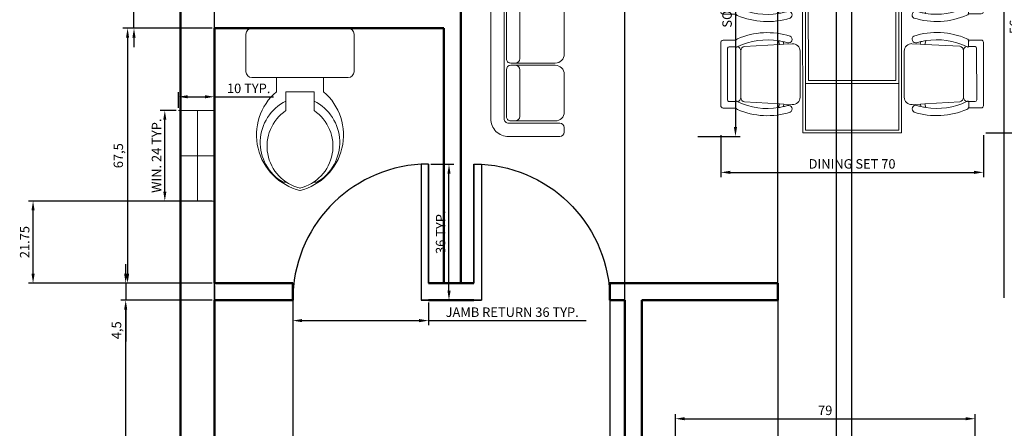
# Model space of a CAD drawing. Units: inches. Extents: x 907 to 2409, y 377 to 1163.
# Tile 2 of 9: x 936 to 1197, y 579 to 687. Entities that reach past the tile are written whole.
import ezdxf

# ---------------------------------------------------------------- set-up
doc = ezdxf.new("R2010")
doc.units = ezdxf.units.IN
for name, color, linetype, lineweight in [('A-ANNO-DIMS', 2, 'Continuous', 18), ('A-DOOR', 3, 'Continuous', 25), ('A-FLOR-FIXT', 9, 'Continuous', 18), ('A-FURN', 8, 'Continuous', 18), ('A-GLAZ', 4, 'Continuous', 18), ('A-WALL', 7, 'Continuous', 50)]:
    doc.layers.add(name, color=color, linetype=linetype, lineweight=lineweight)
doc.styles.get("Standard").update_dxf_attribs({"font": 'arial.ttf'})
doc.dimstyles.new('ISO-25', dxfattribs={"dimtxt": 2.5, "dimasz": 2.5, "dimexe": 1.25, "dimexo": 0.625, "dimtad": 1, "dimtxsty": 'Standard', "dimcen": 2.5, "dimadec": 0, "dimazin": 0, "dimtfac": 1, "dimtmove": 0, "dimatfit": 3, "dimfxl": 1, "dimarcsym": 0})

# ---------------------------------------------------------------- blocks, each defined once
blk = doc.blocks.new('A$C02F3725D')
for p, q in [((0.025, 0.69), (0.435, 0.69)), ((0, 0.505), (0, 0.665)), ((0.46, 0.665), (0.46, 0.505)), ((0.435, 0.48), (0.025, 0.48)), ((0.13, 0.48), (0.13, 0.42)), ((0.33, 0.42), (0.33, 0.48)), ((0.17, 0.34), (0.17, 0.42)), ((0.17, 0.42), (0.29, 0.42)), ((0.29, 0.34), (0.29, 0.42)), ((0.1578, 0.035), (0.1724, 0.035)), ((0.2876, 0.035), (0.3022, 0.035))]:
    blk.add_line(p, q)
for centre, radius, start, end in [((0.025, 0.665), 0.025, 90, 180), ((0.435, 0.665), 0.025, 0, 90), ((0.025, 0.505), 0.025, 180, 270), ((0.435, 0.505), 0.025, 270, 0), ((0.2874, 0.2356), 0.2425, 130.4885, 256.2965), ((0.1726, 0.2356), 0.2425, 283.7035, 49.5115), ((0.2568, 0.2042), 0.196, 116.2742, 239.6668), ((0.2032, 0.2042), 0.196, 300.3332, 63.7258), ((0.2732, 0.1883), 0.1834, 124.2157, 256.394), ((0.1868, 0.1883), 0.1834, 283.606, 55.7843)]:
    blk.add_arc(centre, radius, start, end)
blk = doc.blocks.new('A$C2AFA021D')
for p, q in [((0.8, 2.3), (0.2, 2.3)), ((0.85, 2.2), (0.85, 2.25)), ((0.2, 2.15), (0.8, 2.15)), ((0.225, 2.125), (0.275, 2.125)), ((0.75, 2.125), (0.275, 2.125)), ((0, 2.1), (0, 0.2)), ((0.15, 0.2), (0.15, 2.1)), ((0.175, 1.55), (0.175, 2.075)), ((0.325, 2.075), (0.325, 1.55)), ((0.85, 1.6), (0.85, 2.025)), ((0.275, 1.5), (0.225, 1.5)), ((0.225, 1.475), (0.275, 1.475)), ((0.275, 1.5), (0.75, 1.5)), ((0.75, 1.475), (0.275, 1.475)), ((0.175, 0.875), (0.175, 1.425)), ((0.325, 1.425), (0.325, 0.875)), ((0.85, 0.925), (0.85, 1.375)), ((0.275, 0.825), (0.225, 0.825)), ((0.225, 0.8), (0.275, 0.8)), ((0.275, 0.825), (0.75, 0.825)), ((0.75, 0.8), (0.275, 0.8)), ((0.975, 0.825), (1.4, 0.825)), ((1.625, 0.825), (2.075, 0.825)), ((2.3, 0.825), (2.725, 0.825)), ((2.85, 0.2), (2.85, 0.775)), ((2.9, 0.825), (2.95, 0.825)), ((3, 0.775), (3, 0.2)), ((0.175, 0.225), (0.175, 0.75)), ((0.325, 0.75), (0.325, 0.225)), ((0.85, 0.275), (0.85, 0.7)), ((0.875, 0.275), (0.875, 0.725)), ((1.5, 0.725), (1.5, 0.275)), ((1.525, 0.275), (1.525, 0.725)), ((2.175, 0.725), (2.175, 0.275)), ((2.2, 0.275), (2.2, 0.725)), ((2.825, 0.725), (2.825, 0.275)), ((0.875, 0.275), (0.875, 0.225)), ((1.45, 0.325), (0.925, 0.325)), ((1.5, 0.225), (1.5, 0.275)), ((1.525, 0.275), (1.525, 0.225)), ((2.125, 0.325), (1.575, 0.325)), ((2.175, 0.225), (2.175, 0.275)), ((2.2, 0.275), (2.2, 0.225)), ((2.775, 0.325), (2.25, 0.325)), ((2.825, 0.225), (2.825, 0.275)), ((0.8, 0.15), (0.2, 0.15)), ((0.275, 0.175), (0.225, 0.175)), ((0.275, 0.175), (0.75, 0.175)), ((0.925, 0.175), (1.45, 0.175)), ((0.925, 0.15), (2.8, 0.15)), ((1.575, 0.175), (2.125, 0.175)), ((2.25, 0.175), (2.775, 0.175)), ((0.85, 0), (0.85, 0.1)), ((0.875, 0.1), (0.875, 0)), ((0.2, 0), (0.85, 0)), ((2.8, 0), (0.875, 0))]:
    blk.add_line(p, q)
for centre, radius, start, end in [((0.2, 2.1), 0.2, 90, 180), ((0.8, 2.25), 0.05, 0, 90), ((0.2, 2.1), 0.05, 90, 180), ((0.225, 2.075), 0.05, 90, 180), ((0.275, 2.075), 0.05, 0, 90), ((0.75, 2.025), 0.1, 0, 90), ((0.8, 2.2), 0.05, 270, 0), ((0.225, 1.55), 0.05, 180, 270), ((0.275, 1.55), 0.05, 270, 0), ((0.75, 1.6), 0.1, 270, 0), ((0.225, 1.425), 0.05, 90, 180), ((0.275, 1.425), 0.05, 0, 90), ((0.75, 1.375), 0.1, 360, 90), ((0.75, 0.925), 0.1, 270, 0), ((0.225, 0.875), 0.05, 180, 270), ((0.225, 0.75), 0.05, 90, 180), ((0.275, 0.875), 0.05, 270, 0), ((0.275, 0.75), 0.05, 0, 90), ((0.75, 0.7), 0.1, 0, 90), ((0.975, 0.725), 0.1, 90, 180), ((1.4, 0.725), 0.1, 0, 90), ((1.625, 0.725), 0.1, 90, 180), ((2.075, 0.725), 0.1, 0, 90), ((2.3, 0.725), 0.1, 90, 180), ((2.725, 0.725), 0.1, 0, 90), ((2.9, 0.775), 0.05, 90, 180), ((2.95, 0.775), 0.05, 0, 90), ((0.225, 0.225), 0.05, 180, 270), ((0.275, 0.225), 0.05, 270, 0), ((0.75, 0.275), 0.1, 270, 0), ((0.925, 0.275), 0.05, 90, 180), ((0.925, 0.225), 0.05, 180, 270), ((1.45, 0.275), 0.05, 360, 90), ((1.45, 0.225), 0.05, 270, 0), ((1.575, 0.275), 0.05, 90, 180), ((1.575, 0.225), 0.05, 180, 270), ((2.125, 0.275), 0.05, 360, 90), ((2.125, 0.225), 0.05, 270, 0), ((2.25, 0.275), 0.05, 90, 180), ((2.25, 0.225), 0.05, 180, 270), ((2.775, 0.275), 0.05, 360, 90), ((2.775, 0.225), 0.05, 270, 0), ((0.2, 0.2), 0.2, 180, 270), ((0.2, 0.2), 0.05, 180, 270), ((0.8, 0.1), 0.05, 0, 90), ((0.925, 0.1), 0.05, 90, 180), ((2.8, 0.2), 0.2, 270, 0), ((2.8, 0.2), 0.05, 270, 0)]:
    blk.add_arc(centre, radius, start, end)
blk = doc.blocks.new('A$C7D96336B')
for p, q in [((280, 0.2), (-280, -0.2)), ((280.8, -1199.8), (280, 0.2)), ((-280, -0.2), (-279.2, -1200.2)), ((264, -15.8), (-264, -16.2)), ((-264, -16.2), (-263.2, -1184.2)), ((264.8, -1183.8), (264, -15.8)), ((-742.8, -515.1), (-743.2, -156.2)), ((-658.1, -143.4), (-730.7, -143.6)), ((-659.8, -143.4), (-659.7, -178.7)), ((-416.5, -146.3), (-411.5, -167.3)), ((-386.1, -165.8), (-411.5, -167.3)), ((-389.5, -151.7), (-386.1, -165.8)), ((-338.9, -163.1), (-386.1, -165.8)), ((339.1, -162.6), (386.3, -165.3)), ((389.7, -151.1), (386.3, -165.3)), ((386.3, -165.3), (411.7, -166.7)), ((416.7, -145.7), (411.7, -166.7)), ((411.7, -166.7), (609.3, -177.8)), ((658.3, -142.5), (730.9, -142.6)), ((659.9, -142.6), (659.9, -177.8)), ((743.5, -514.1), (743.4, -155.2)), ((-704.9, -188.8), (-704.6, -482.3)), ((-659.3, -180.3), (-696.6, -180.5)), ((-629.9, -467.6), (-630.2, -203.4)), ((-411.5, -167.3), (-609.1, -178.7)), ((-294.5, -465.7), (-294.4, -204.7)), ((295.2, -465.3), (294.7, -204.3)), ((630.5, -466.8), (630.5, -202.5)), ((659.5, -179.5), (696.9, -179.5)), ((705.2, -187.9), (705.3, -481.4)), ((-263.8, -280.2), (264.2, -279.8)), ((-263.8, -280.2), (264.2, -279.8)), ((-263.4, -920.2), (-263.8, -280.2)), ((-247.8, -296.2), (248.2, -295.8)), ((-247.4, -904.2), (-247.8, -296.2)), ((248.2, -295.8), (248.6, -903.8)), ((264.2, -279.8), (264.6, -919.8)), ((-659, -490.7), (-696.3, -490.7)), ((-659.4, -522.3), (-659.3, -492.4)), ((-411.1, -503.3), (-608.7, -492.3)), ((411.8, -502.7), (609.4, -491.4)), ((659.6, -489.8), (697, -489.7)), ((660.1, -521.4), (660, -491.5)), ((-657.7, -527.6), (-730.3, -527.6)), ((-416.1, -524.3), (-411.1, -503.3)), ((-385.8, -504.7), (-411.1, -503.3)), ((-389.1, -518.8), (-385.8, -504.7)), ((-338.5, -507.3), (-385.8, -504.7)), ((339.2, -506.9), (386.5, -504.2)), ((386.5, -504.2), (411.8, -502.7)), ((389.8, -518.3), (386.5, -504.2)), ((416.8, -523.7), (411.8, -502.7)), ((658.4, -526.7), (731, -526.6)), ((-742.7, -688.4), (-742.6, -1047.3)), ((-657.6, -675.8), (-730.2, -675.9)), ((-704.4, -1014.6), (-704.5, -721.1)), ((-658.8, -712.7), (-696.2, -712.8)), ((-659.3, -681), (-659.2, -711)), ((-411, -699.8), (-608.6, -711)), ((-416, -678.8), (-411, -699.8)), ((-385.6, -698.3), (-411, -699.8)), ((-389, -684.2), (-385.6, -698.3)), ((-338.4, -695.6), (-385.6, -698.3)), ((339.3, -695.2), (386.6, -697.8)), ((389.9, -683.7), (386.6, -697.8)), ((386.6, -697.8), (411.9, -699.2)), ((416.9, -678.2), (411.9, -699.2)), ((411.9, -699.2), (609.5, -710.2)), ((658.5, -674.9), (731.1, -674.9)), ((659.8, -711.8), (697.1, -711.8)), ((660.2, -680.2), (660.2, -710.1)), ((705.8, -1013.7), (705.5, -720.2)), ((743.6, -687.4), (744, -1046.3)), ((-629.7, -735.7), (-629.6, -1000)), ((-294.4, -737.1), (-293.9, -998.2)), ((295.3, -736.7), (295.2, -997.8)), ((630.7, -734.9), (631, -999.1)), ((264.6, -919.8), (-263.4, -920.2)), ((248.6, -903.8), (-247.4, -904.2)), ((-658.7, -1023), (-696.1, -1023)), ((-659.1, -1059.9), (-659.1, -1024.7)), ((-410.9, -1035.8), (-608.5, -1024.6)), ((-415.9, -1056.8), (-410.9, -1035.8)), ((-385.5, -1037.2), (-410.9, -1035.8)), ((-388.9, -1051.4), (-385.5, -1037.2)), ((-338.3, -1039.9), (-385.5, -1037.2)), ((339.7, -1039.4), (386.9, -1036.7)), ((386.9, -1036.7), (412.3, -1035.2)), ((390.3, -1050.8), (386.9, -1036.7)), ((412.3, -1035.2), (609.9, -1023.8)), ((417.3, -1056.2), (412.3, -1035.2)), ((658.9, -1059), (731.5, -1058.9)), ((660.1, -1022.1), (697.4, -1022)), ((660.6, -1059), (660.5, -1023.8)), ((-657.5, -1059.9), (-730.1, -1059.9)), ((-279.2, -1200.2), (280.8, -1199.8)), ((-263.2, -1184.2), (264.8, -1183.8))]:
    blk.add_line(p, q)
for centre, radius, start, end in [((-478.6, -532.7), 432.3, 72.7119, 113.3258), ((479.4, -532), 432.3, 66.7517, 107.3656), ((-730.7, -156.1), 12.5, 141.7605, 180.1459), ((-730.7, -156.1), 12.5, 90.1463, 141.7605), ((-643.2, -151), 16.7, 153.004, 184.8567), ((-643.2, -151), 16.7, 113.3258, 153.004), ((-479.1, -531.9), 390.7, 80.7703, 115.5809), ((-479.1, -531.9), 390.7, 76.7336, 80.7703), ((-479.1, -531.9), 390.7, 73.1676, 76.7336), ((-360.6, -137.9), 20.8, 254.7795, 60.0186), ((-336.5, -204.7), 41.7, 0.1463, 93.3068), ((336.7, -204.2), 41.7, 86.7707, 179.9312), ((360.7, -137.4), 20.8, 120.0589, 285.298), ((479.9, -531.2), 390.7, 103.3439, 106.9099), ((479.9, -531.2), 390.7, 99.3072, 103.3439), ((479.9, -531.2), 390.7, 64.4966, 99.3072), ((643.4, -150.1), 16.7, 27.0735, 66.7517), ((643.4, -150.1), 16.7, 355.2209, 27.0735), ((730.9, -155.1), 12.5, 38.317, 89.9312), ((730.9, -155.1), 12.5, 359.9316, 38.317), ((-696.6, -188.8), 8.33, 90.1463, 180.1463), ((-655.5, -178.6), 4.17, 180.1463, 296.5296), ((-479.1, -531.9), 390.7, 115.5809, 116.5296), ((-655.2, -203.4), 25, 0.1463, 72.8968), ((-605.2, -203.4), 25, 98.9209, 179.9714), ((605.5, -202.6), 25, 0.1061, 81.1566), ((655.5, -202.5), 25, 107.1807, 179.9312), ((479.9, -531.2), 390.7, 63.5479, 64.4966), ((655.7, -177.8), 4.17, 243.5479, 359.9312), ((696.9, -187.8), 8.33, 359.9312, 89.9312), ((-696.3, -482.3), 8.33, 179.9714, 269.9714), ((-655.2, -492.4), 4.17, 63.5881, 179.9714), ((-479.5, -138.8), 390.7, 243.5881, 244.5368), ((-654.9, -467.6), 25, 287.2209, 359.9714), ((-479.5, -138.8), 390.7, 244.5368, 279.3474), ((-604.9, -467.6), 25, 180.1463, 261.1967), ((-336.2, -465.7), 41.7, 266.8108, 359.9714), ((336.8, -465.3), 41.7, 180.1061, 273.2667), ((479.7, -138.1), 390.7, 260.7301, 295.5407), ((605.5, -466.7), 25, 278.8808, 359.9312), ((655.5, -466.7), 25, 180.1061, 252.8566), ((479.7, -138.1), 390.7, 295.5407, 296.4894), ((655.8, -491.5), 4.17, 0.1061, 116.4894), ((697, -481.4), 8.33, 270.1061, 0.1061), ((-730.3, -515.1), 12.5, 179.9717, 218.3572), ((-730.3, -515.1), 12.5, 218.3572, 269.9714), ((-642.9, -520), 16.7, 175.261, 207.1136), ((-642.9, -520), 16.7, 207.1136, 246.7919), ((-479.1, -138), 432.3, 246.7919, 287.4058), ((-479.5, -138.8), 390.7, 279.3474, 283.3841), ((-479.5, -138.8), 390.7, 283.3841, 286.9501), ((-360.2, -532.5), 20.8, 300.0991, 105.3382), ((360.9, -532), 20.8, 74.7393, 239.9785), ((479.2, -137.3), 432.3, 252.6717, 293.2857), ((479.7, -138.1), 390.7, 253.1274, 256.6934), ((479.7, -138.1), 390.7, 256.6934, 260.7301), ((643.6, -519.1), 16.7, 293.2857, 332.9639), ((643.6, -519.1), 16.7, 332.9639, 4.8165), ((731, -514.1), 12.5, 270.1061, 321.7203), ((731, -514.1), 12.5, 321.7203, 0.1058), ((-642.7, -683.3), 16.7, 113.2857, 152.9639), ((-478.4, -1065.1), 432.3, 72.6717, 113.2857), ((-360.1, -670.4), 20.8, 254.7393, 59.9785), ((361, -670), 20.8, 120.0991, 285.3382), ((479.9, -1064.5), 432.3, 66.7919, 107.4058), ((643.7, -682.5), 16.7, 27.1136, 66.7919), ((-730.2, -688.4), 12.5, 141.7203, 180.1058), ((-730.2, -688.4), 12.5, 90.1061, 141.7203), ((-696.1, -721.1), 8.33, 90.1061, 180.1061), ((-642.7, -683.3), 16.7, 152.9639, 184.8165), ((-655, -711), 4.17, 180.1061, 296.4894), ((-478.9, -1064.3), 390.7, 115.5407, 116.4894), ((-478.9, -1064.3), 390.7, 80.7301, 115.5407), ((-654.7, -735.8), 25, 0.1061, 72.8566), ((-604.7, -735.7), 25, 98.8808, 179.9312), ((-478.9, -1064.3), 390.7, 76.6934, 80.7301), ((-478.9, -1064.3), 390.7, 73.1274, 76.6934), ((-336, -737.2), 41.7, 0.1061, 93.2667), ((337, -736.8), 41.7, 86.8108, 179.9714), ((480.4, -1063.7), 390.7, 103.3841, 106.9501), ((480.4, -1063.7), 390.7, 99.3474, 103.3841), ((480.4, -1063.7), 390.7, 64.5368, 99.3474), ((605.7, -734.9), 25, 0.1463, 81.1967), ((655.7, -734.9), 25, 107.2209, 179.9714), ((480.4, -1063.7), 390.7, 63.5881, 64.5368), ((656, -710.1), 4.17, 243.5881, 359.9714), ((643.7, -682.5), 16.7, 355.261, 27.1136), ((697.1, -720.1), 8.33, 359.9714, 89.9714), ((731.1, -687.4), 12.5, 38.3572, 89.9714), ((731.1, -687.4), 12.5, 359.9717, 38.3572), ((-654.6, -1000), 25, 287.1807, 359.9312), ((-604.6, -999.9), 25, 180.1061, 261.1566), ((-335.9, -998.3), 41.7, 266.7707, 359.9312), ((337.3, -997.8), 41.7, 180.1463, 273.3068), ((606, -999.1), 25, 278.9209, 359.9714), ((656, -999.1), 25, 180.1463, 252.8968), ((-730.1, -1047.4), 12.5, 179.9316, 218.317), ((-730.1, -1047.4), 12.5, 218.317, 269.9312), ((-696.1, -1014.6), 8.33, 179.9312, 269.9312), ((-642.6, -1052.4), 16.7, 175.2209, 207.0735), ((-654.9, -1024.7), 4.17, 63.5479, 179.9312), ((-479.1, -671.2), 390.7, 243.5479, 244.4966), ((-479.1, -671.2), 390.7, 244.4966, 279.3072), ((-479.1, -671.2), 390.7, 279.3072, 283.3439), ((-479.1, -671.2), 390.7, 283.3439, 286.9099), ((-359.9, -1065.1), 20.8, 300.0589, 105.298), ((361.4, -1064.6), 20.8, 74.7795, 240.0186), ((480, -670.6), 390.7, 253.1676, 256.7336), ((480, -670.6), 390.7, 256.7336, 260.7703), ((480, -670.6), 390.7, 260.7703, 295.5809), ((480, -670.6), 390.7, 295.5809, 296.5296), ((644, -1051.5), 16.7, 293.3258, 333.004), ((656.3, -1023.8), 4.17, 0.1463, 116.5296), ((644, -1051.5), 16.7, 333.004, 4.8567), ((697.4, -1013.7), 8.33, 270.1463, 0.1463), ((731.5, -1046.4), 12.5, 270.1463, 321.7605), ((731.5, -1046.4), 12.5, 321.7605, 0.1459), ((-642.6, -1052.4), 16.7, 207.0735, 246.7517), ((-478.6, -670.4), 432.3, 246.7517, 287.3656), ((479.5, -669.8), 432.3, 252.7119, 293.3258)]:
    blk.add_arc(centre, radius, start, end)
blk = doc.blocks.new('*D34')
at = {"layer": 'A-ANNO-DIMS', "color": 0, "lineweight": -2, "transparency": 16777216}
for p, q in [((966.32, 691.62), (966.32, 700.04)), ((986.99, 689.12), (965.07, 689.12)), ((966.32, 684.62), (966.32, 689.12)), ((986.99, 684.62), (965.07, 684.62)), ((966.32, 682.12), (966.32, 679.62))]:
    blk.add_line(p, q, dxfattribs=at)
at = {"layer": 'A-ANNO-DIMS', "color": 0, "transparency": 16777216}
for points in [[(965.9, 691.62), (966.74, 691.62), (966.32, 689.12)], [(965.9, 682.12), (966.74, 682.12), (966.32, 684.62)]]:
    blk.add_solid(points, dxfattribs=at)
at = {"layer": 'Defpoints', "color": 0, "transparency": 16777216}
for p in [(966.32, 689.12), (987.61, 689.12), (987.61, 684.62)]:
    blk.add_point(p, dxfattribs=at)
at = {"layer": 'A-ANNO-DIMS', "color": 0, "transparency": 16777216, "insert": (964.2, 697.08), "char_height": 2.5, "attachment_point": 5, "rotation": 90}
blk.add_mtext('4,5', dxfattribs=at)
blk = doc.blocks.new('*D35')
at = {"layer": 'A-ANNO-DIMS', "color": 0, "lineweight": -2, "transparency": 16777216}
for p, q in [((986.99, 684.62), (963.37, 684.62)), ((964.62, 682.12), (964.62, 619.62)), ((986.99, 617.12), (963.37, 617.12))]:
    blk.add_line(p, q, dxfattribs=at)
at = {"layer": 'A-ANNO-DIMS', "color": 0, "transparency": 16777216}
for points in [[(964.2, 682.12), (965.03, 682.12), (964.62, 684.62)], [(964.2, 619.62), (965.03, 619.62), (964.62, 617.12)]]:
    blk.add_solid(points, dxfattribs=at)
at = {"layer": 'Defpoints', "color": 0, "transparency": 16777216}
for p in [(987.61, 684.62), (964.62, 617.12), (987.61, 617.12)]:
    blk.add_point(p, dxfattribs=at)
at = {"layer": 'A-ANNO-DIMS', "color": 0, "transparency": 16777216, "insert": (962.49, 650.87), "char_height": 2.5, "attachment_point": 5, "rotation": 90}
blk.add_mtext('67,5', dxfattribs=at)
blk = doc.blocks.new('*D36')
at = {"layer": 'A-ANNO-DIMS', "color": 0, "lineweight": -2, "transparency": 16777216}
for p, q in [((964.12, 619.62), (964.12, 622.12)), ((986.99, 617.12), (962.87, 617.12)), ((964.12, 617.12), (964.12, 612.62)), ((986.99, 612.62), (962.87, 612.62)), ((964.12, 610.12), (964.12, 601.7))]:
    blk.add_line(p, q, dxfattribs=at)
at = {"layer": 'A-ANNO-DIMS', "color": 0, "transparency": 16777216}
for points in [[(963.7, 619.62), (964.53, 619.62), (964.12, 617.12)], [(963.7, 610.12), (964.53, 610.12), (964.12, 612.62)]]:
    blk.add_solid(points, dxfattribs=at)
at = {"layer": 'Defpoints', "color": 0, "transparency": 16777216}
for p in [(987.61, 617.12), (964.12, 612.62), (987.61, 612.62)]:
    blk.add_point(p, dxfattribs=at)
at = {"layer": 'A-ANNO-DIMS', "color": 0, "transparency": 16777216, "insert": (962, 604.66), "char_height": 2.5, "attachment_point": 5, "rotation": 90}
blk.add_mtext('4,5', dxfattribs=at)
blk = doc.blocks.new('*D37')
at = {"layer": 'A-ANNO-DIMS', "color": 0, "lineweight": -2, "transparency": 16777216}
for p, q in [((986.99, 612.62), (962.87, 612.62)), ((964.12, 428.37), (964.12, 610.12)), ((986.99, 425.87), (962.87, 425.87))]:
    blk.add_line(p, q, dxfattribs=at)
at = {"layer": 'A-ANNO-DIMS', "color": 0, "transparency": 16777216}
for points in [[(963.7, 610.12), (964.53, 610.12), (964.12, 612.62)], [(963.7, 428.37), (964.53, 428.37), (964.12, 425.87)]]:
    blk.add_solid(points, dxfattribs=at)
at = {"layer": 'Defpoints', "color": 0, "transparency": 16777216}
for p in [(964.12, 612.62), (987.61, 612.62), (987.61, 425.87)]:
    blk.add_point(p, dxfattribs=at)
at = {"layer": 'A-ANNO-DIMS', "color": 0, "transparency": 16777216, "insert": (961.99, 519.25), "char_height": 2.5, "attachment_point": 5, "rotation": 90}
blk.add_mtext('186,75', dxfattribs=at)
blk = doc.blocks.new('WIN-24IN')
for p, q in [((0.53, 23.99), (0, 23.99)), ((9.53, 24), (0.53, 24)), ((5.03, 0), (5.03, 24)), ((9.53, 12), (0.53, 12)), ((9.53, 0), (0.53, 0))]:
    blk.add_line(p, q)
blk = doc.blocks.new('DOOR-36IN-JAMB-RETURN')
for p, q in [((36, 36), (36, 4.5)), ((36, 0), (34, 0)), ((36, 0), (34, 0))]:
    blk.add_line(p, q)
blk.add_lwpolyline([(36, 4.5), (36, 36), (34, 36), (34, 0), (36, 0)])
blk.add_arc((36.06, 0), 36.06, 93.2732, 180)
blk = doc.blocks.new('*D45')
at = {"layer": 'A-ANNO-DIMS', "color": 0, "lineweight": -2, "transparency": 16777216}
for p, q in [((1008.36, 612), (1008.36, 605.97)), ((1044.36, 612), (1044.36, 605.97)), ((1010.86, 607.22), (1041.86, 607.22)), ((1044.36, 607.22), (1086.14, 607.22))]:
    blk.add_line(p, q, dxfattribs=at)
at = {"layer": 'A-ANNO-DIMS', "color": 0, "transparency": 16777216}
for points in [[(1010.86, 607.64), (1010.86, 606.8), (1008.36, 607.22)], [(1041.86, 607.64), (1041.86, 606.8), (1044.36, 607.22)]]:
    blk.add_solid(points, dxfattribs=at)
at = {"layer": 'Defpoints', "color": 0, "transparency": 16777216}
for p in [(1008.36, 612.62), (1044.36, 612.62), (1044.36, 607.22)]:
    blk.add_point(p, dxfattribs=at)
at = {"layer": 'A-ANNO-DIMS', "color": 0, "transparency": 16777216, "insert": (1066.5, 609.12), "char_height": 2.5, "attachment_point": 5}
blk.add_mtext('JAMB RETURN 36 TYP.', dxfattribs=at)
blk = doc.blocks.new('*D46')
at = {"layer": 'A-ANNO-DIMS', "color": 0, "lineweight": -2, "transparency": 16777216}
for p, q in [((1044.99, 648.62), (1051.01, 648.62)), ((1049.76, 615.12), (1049.76, 646.12)), ((1044.99, 612.62), (1051.01, 612.62))]:
    blk.add_line(p, q, dxfattribs=at)
at = {"layer": 'A-ANNO-DIMS', "color": 0, "transparency": 16777216}
for points in [[(1049.35, 646.12), (1050.18, 646.12), (1049.76, 648.62)], [(1049.35, 615.12), (1050.18, 615.12), (1049.76, 612.62)]]:
    blk.add_solid(points, dxfattribs=at)
at = {"layer": 'Defpoints', "color": 0, "transparency": 16777216}
for p in [(1044.36, 648.62), (1049.76, 648.62), (1044.36, 612.62)]:
    blk.add_point(p, dxfattribs=at)
at = {"layer": 'A-ANNO-DIMS', "color": 0, "transparency": 16777216, "insert": (1047.86, 630.62), "char_height": 2.5, "attachment_point": 5, "rotation": 90}
blk.add_mtext('36 TYP.', dxfattribs=at)
blk = doc.blocks.new('*D47')
at = {"layer": 'A-ANNO-DIMS', "color": 0, "lineweight": -2, "transparency": 16777216}
for p, q in [((977.46, 662.87), (973.23, 662.87)), ((974.48, 641.37), (974.48, 660.37)), ((977.46, 638.87), (973.23, 638.87))]:
    blk.add_line(p, q, dxfattribs=at)
at = {"layer": 'A-ANNO-DIMS', "color": 0, "transparency": 16777216}
for points in [[(974.07, 660.37), (974.9, 660.37), (974.48, 662.87)], [(974.07, 641.37), (974.9, 641.37), (974.48, 638.87)]]:
    blk.add_solid(points, dxfattribs=at)
at = {"layer": 'Defpoints', "color": 0, "transparency": 16777216}
for p in [(974.48, 662.87), (978.08, 662.87), (978.08, 638.87)]:
    blk.add_point(p, dxfattribs=at)
at = {"layer": 'A-ANNO-DIMS', "color": 0, "transparency": 16777216, "insert": (972.6, 650.87), "char_height": 2.5, "attachment_point": 5, "rotation": 90}
blk.add_mtext('WIN. 24 TYP.', dxfattribs=at)
blk = doc.blocks.new('*D48')
at = {"layer": 'A-ANNO-DIMS', "color": 0, "lineweight": -2, "transparency": 16777216}
for p, q in [((978.08, 663.5), (978.08, 667.72)), ((987.61, 663.5), (987.61, 667.72)), ((980.58, 666.47), (985.11, 666.47)), ((987.61, 666.47), (1003.3, 666.47))]:
    blk.add_line(p, q, dxfattribs=at)
at = {"layer": 'A-ANNO-DIMS', "color": 0, "transparency": 16777216}
for points in [[(980.58, 666.89), (980.58, 666.05), (978.08, 666.47)], [(985.11, 666.89), (985.11, 666.05), (987.61, 666.47)]]:
    blk.add_solid(points, dxfattribs=at)
at = {"layer": 'Defpoints', "color": 0, "transparency": 16777216}
for p in [(987.61, 666.47), (978.08, 662.87), (987.61, 662.87)]:
    blk.add_point(p, dxfattribs=at)
at = {"layer": 'A-ANNO-DIMS', "color": 0, "transparency": 16777216, "insert": (996.7, 668.37), "char_height": 2.5, "attachment_point": 5}
blk.add_mtext('10 TYP.', dxfattribs=at)
blk = doc.blocks.new('*D53')
at = {"layer": 'A-ANNO-DIMS', "color": 0, "lineweight": -2, "transparency": 16777216}
for p, q in [((1115.67, 726.66), (1126.9, 726.66)), ((1125.65, 724.16), (1125.65, 658.44)), ((1115.67, 655.94), (1126.9, 655.94))]:
    blk.add_line(p, q, dxfattribs=at)
at = {"layer": 'A-ANNO-DIMS', "color": 0, "transparency": 16777216}
for points in [[(1125.24, 724.16), (1126.07, 724.16), (1125.65, 726.66)], [(1125.24, 658.44), (1126.07, 658.44), (1125.65, 655.94)]]:
    blk.add_solid(points, dxfattribs=at)
at = {"layer": 'Defpoints', "color": 0, "transparency": 16777216}
for p in [(1115.05, 726.66), (1115.05, 655.94), (1125.65, 655.94)]:
    blk.add_point(p, dxfattribs=at)
at = {"layer": 'A-ANNO-DIMS', "color": 0, "transparency": 16777216, "insert": (1123.74, 691.3), "char_height": 2.5, "attachment_point": 5, "rotation": 90}
blk.add_mtext('SOFA 71', dxfattribs=at)
blk = doc.blocks.new('*D56')
at = {"layer": 'A-ANNO-DIMS', "color": 0, "lineweight": -2, "transparency": 16777216}
for p, q in [((1109.72, 566.33), (1109.72, 582.49)), ((1189.13, 566.33), (1189.13, 582.49)), ((1112.22, 581.24), (1186.63, 581.24))]:
    blk.add_line(p, q, dxfattribs=at)
at = {"layer": 'A-ANNO-DIMS', "color": 0, "transparency": 16777216}
for points in [[(1112.22, 581.66), (1112.22, 580.83), (1109.72, 581.24)], [(1186.63, 581.66), (1186.63, 580.83), (1189.13, 581.24)]]:
    blk.add_solid(points, dxfattribs=at)
at = {"layer": 'Defpoints', "color": 0, "transparency": 16777216}
for p in [(1189.13, 581.24), (1109.72, 565.7), (1189.13, 565.7)]:
    blk.add_point(p, dxfattribs=at)
at = {"layer": 'A-ANNO-DIMS', "color": 0, "transparency": 16777216, "insert": (1149.42, 583.14), "char_height": 2.5, "attachment_point": 5}
blk.add_mtext('79', dxfattribs=at)
blk = doc.blocks.new('*D57')
at = {"layer": 'A-ANNO-DIMS', "color": 0, "lineweight": -2, "transparency": 16777216}
for p, q in [((1121.75, 656.27), (1121.75, 645.21)), ((1191.34, 656.27), (1191.34, 645.21)), ((1124.25, 646.46), (1188.84, 646.46))]:
    blk.add_line(p, q, dxfattribs=at)
at = {"layer": 'A-ANNO-DIMS', "color": 0, "transparency": 16777216}
for points in [[(1124.25, 646.88), (1124.25, 646.04), (1121.75, 646.46)], [(1188.84, 646.88), (1188.84, 646.04), (1191.34, 646.46)]]:
    blk.add_solid(points, dxfattribs=at)
at = {"layer": 'Defpoints', "color": 0, "transparency": 16777216}
for p in [(1121.75, 656.9), (1191.34, 656.9), (1191.34, 646.46)]:
    blk.add_point(p, dxfattribs=at)
at = {"layer": 'A-ANNO-DIMS', "color": 0, "transparency": 16777216, "insert": (1156.54, 648.38), "char_height": 2.5, "attachment_point": 5}
blk.add_mtext('DINING SET 70', dxfattribs=at)
blk = doc.blocks.new('*D58')
at = {"layer": 'A-ANNO-DIMS', "color": 0, "lineweight": -2, "transparency": 16777216}
for p, q in [((1191.96, 713.06), (1203.02, 713.06)), ((1201.77, 659.4), (1201.77, 710.56)), ((1191.96, 656.9), (1203.02, 656.9))]:
    blk.add_line(p, q, dxfattribs=at)
at = {"layer": 'A-ANNO-DIMS', "color": 0, "transparency": 16777216}
for points in [[(1201.36, 710.56), (1202.19, 710.56), (1201.77, 713.06)], [(1201.36, 659.4), (1202.19, 659.4), (1201.77, 656.9)]]:
    blk.add_solid(points, dxfattribs=at)
at = {"layer": 'Defpoints', "color": 0, "transparency": 16777216}
for p in [(1191.34, 713.06), (1201.77, 713.06), (1191.34, 656.9)]:
    blk.add_point(p, dxfattribs=at)
at = {"layer": 'A-ANNO-DIMS', "color": 0, "transparency": 16777216, "insert": (1199.87, 684.98), "char_height": 2.5, "attachment_point": 5, "rotation": 90}
blk.add_mtext('56', dxfattribs=at)
blk = doc.blocks.new('*D62')
at = {"layer": 'A-ANNO-DIMS', "color": 0, "lineweight": -2, "transparency": 16777216}
for p, q in [((987.61, 426.5), (987.61, 1056.62)), ((1096.36, 426.5), (1096.36, 1056.62)), ((990.11, 1055.37), (1093.86, 1055.37))]:
    blk.add_line(p, q, dxfattribs=at)
at = {"layer": 'A-ANNO-DIMS', "color": 0, "transparency": 16777216}
for points in [[(990.11, 1055.79), (990.11, 1054.95), (987.61, 1055.37)], [(1093.86, 1055.79), (1093.86, 1054.95), (1096.36, 1055.37)]]:
    blk.add_solid(points, dxfattribs=at)
at = {"layer": 'Defpoints', "color": 0, "transparency": 16777216}
for p in [(1096.36, 1055.37), (987.61, 425.87), (1096.36, 425.87)]:
    blk.add_point(p, dxfattribs=at)
at = {"layer": 'A-ANNO-DIMS', "color": 0, "transparency": 16777216, "insert": (1041.99, 1057.27), "char_height": 2.5, "attachment_point": 5}
blk.add_mtext('108.75', dxfattribs=at)
blk = doc.blocks.new('*D72')
at = {"layer": 'A-ANNO-DIMS', "color": 0, "lineweight": -2, "transparency": 16777216}
for p, q in [((986.99, 638.87), (938.33, 638.87)), ((939.58, 619.62), (939.58, 636.37)), ((986.99, 617.12), (938.33, 617.12))]:
    blk.add_line(p, q, dxfattribs=at)
at = {"layer": 'A-ANNO-DIMS', "color": 0, "transparency": 16777216}
for points in [[(939.17, 636.37), (940, 636.37), (939.58, 638.87)], [(939.17, 619.62), (940, 619.62), (939.58, 617.12)]]:
    blk.add_solid(points, dxfattribs=at)
at = {"layer": 'Defpoints', "color": 0, "transparency": 16777216}
for p in [(939.58, 638.87), (987.61, 638.87), (987.61, 617.12)]:
    blk.add_point(p, dxfattribs=at)
at = {"layer": 'A-ANNO-DIMS', "color": 0, "transparency": 16777216, "insert": (937.68, 628), "char_height": 2.5, "attachment_point": 5, "rotation": 90}
blk.add_mtext('21.75', dxfattribs=at)
blk = doc.blocks.new('*D75')
at = {"layer": 'A-ANNO-DIMS', "color": 0, "lineweight": -2, "transparency": 16777216}
for p, q in [((1136.86, 613.25), (1136.86, 1056.62)), ((1196.86, 613.25), (1196.86, 1056.62)), ((1139.36, 1055.37), (1194.36, 1055.37))]:
    blk.add_line(p, q, dxfattribs=at)
at = {"layer": 'A-ANNO-DIMS', "color": 0, "transparency": 16777216}
for points in [[(1139.36, 1055.79), (1139.36, 1054.95), (1136.86, 1055.37)], [(1194.36, 1055.79), (1194.36, 1054.95), (1196.86, 1055.37)]]:
    blk.add_solid(points, dxfattribs=at)
at = {"layer": 'Defpoints', "color": 0, "transparency": 16777216}
for p in [(1196.86, 1055.37), (1136.86, 612.62), (1196.86, 612.62)]:
    blk.add_point(p, dxfattribs=at)
at = {"layer": 'A-ANNO-DIMS', "color": 0, "transparency": 16777216, "insert": (1166.86, 1057.27), "char_height": 2.5, "attachment_point": 5}
blk.add_mtext('60', dxfattribs=at)
blk = doc.blocks.new('*D82')
at = {"layer": 'A-ANNO-DIMS', "color": 0, "lineweight": -2, "transparency": 16777216}
for p, q in [((987.61, 616.5), (987.61, 377.12)), ((1008.36, 616.5), (1008.36, 377.12)), ((990.11, 378.37), (1005.86, 378.37))]:
    blk.add_line(p, q, dxfattribs=at)
at = {"layer": 'A-ANNO-DIMS', "color": 0, "transparency": 16777216}
for points in [[(990.11, 378.79), (990.11, 377.95), (987.61, 378.37)], [(1005.86, 378.79), (1005.86, 377.95), (1008.36, 378.37)]]:
    blk.add_solid(points, dxfattribs=at)
at = {"layer": 'Defpoints', "color": 0, "transparency": 16777216}
for p in [(987.61, 617.12), (1008.36, 617.12), (1008.36, 378.37)]:
    blk.add_point(p, dxfattribs=at)
at = {"layer": 'A-ANNO-DIMS', "color": 0, "transparency": 16777216, "insert": (997.99, 380.27), "char_height": 2.5, "attachment_point": 5}
blk.add_mtext('20.75', dxfattribs=at)
blk = doc.blocks.new('*D83')
at = {"layer": 'A-ANNO-DIMS', "color": 0, "lineweight": -2, "transparency": 16777216}
for p, q in [((1092.36, 616.5), (1092.36, 377.12)), ((1136.86, 616.5), (1136.86, 377.12)), ((1094.86, 378.37), (1134.36, 378.37))]:
    blk.add_line(p, q, dxfattribs=at)
at = {"layer": 'A-ANNO-DIMS', "color": 0, "transparency": 16777216}
for points in [[(1094.86, 378.79), (1094.86, 377.95), (1092.36, 378.37)], [(1134.36, 378.79), (1134.36, 377.95), (1136.86, 378.37)]]:
    blk.add_solid(points, dxfattribs=at)
at = {"layer": 'Defpoints', "color": 0, "transparency": 16777216}
for p in [(1092.36, 617.12), (1136.86, 617.12), (1136.86, 378.37)]:
    blk.add_point(p, dxfattribs=at)
at = {"layer": 'A-ANNO-DIMS', "color": 0, "transparency": 16777216, "insert": (1114.61, 380.27), "char_height": 2.5, "attachment_point": 5}
blk.add_mtext('44.5', dxfattribs=at)
blk = doc.blocks.new('*D84')
at = {"layer": 'A-ANNO-DIMS', "color": 0, "lineweight": -2, "transparency": 16777216}
for p, q in [((1152.36, 772.5), (1152.36, 377.12)), ((1156.36, 772.5), (1156.36, 377.12)), ((1149.86, 378.37), (1147.36, 378.37)), ((1152.36, 378.37), (1156.36, 378.37)), ((1158.86, 378.37), (1161.36, 378.37))]:
    blk.add_line(p, q, dxfattribs=at)
at = {"layer": 'A-ANNO-DIMS', "color": 0, "transparency": 16777216}
for points in [[(1149.86, 378.79), (1149.86, 377.95), (1152.36, 378.37)], [(1158.86, 378.79), (1158.86, 377.95), (1156.36, 378.37)]]:
    blk.add_solid(points, dxfattribs=at)
at = {"layer": 'Defpoints', "color": 0, "transparency": 16777216}
for p in [(1152.36, 773.12), (1156.36, 773.12), (1156.36, 378.37)]:
    blk.add_point(p, dxfattribs=at)
at = {"layer": 'A-ANNO-DIMS', "color": 0, "transparency": 16777216, "insert": (1154.36, 380.25), "char_height": 2.5, "attachment_point": 5}
blk.add_mtext('4', dxfattribs=at)

msp = doc.modelspace()

# ---------------------------------------------------------------- linework, layer by layer
at = {"layer": 'A-WALL'}
for p, q in [((978.6122, 1016.8705), (978.6122, 416.8705)), ((1052.8622, 728.6205), (1052.8622, 617.1205)), ((987.6122, 684.6205), (1048.3622, 684.6205)), ((987.6122, 684.6205), (987.6122, 617.1205)), ((1048.3622, 684.6205), (1048.3622, 617.1205)), ((987.6122, 617.1205), (1008.3622, 617.1205)), ((1008.3622, 617.1205), (1008.3622, 612.6205)), ((1044.3622, 617.1205), (1056.3622, 617.1205)), ((1092.3622, 612.6205), (1092.3622, 617.1205)), ((1092.3622, 617.1205), (1136.8622, 617.1205)), ((1136.8622, 612.6205), (1136.8622, 617.1205)), ((978.6122, 614.8705), (978.6122, 416.8705)), ((987.6122, 612.6205), (1008.3622, 612.6205)), ((987.6122, 612.6205), (987.6122, 425.8705)), ((1044.3622, 612.6205), (1056.3622, 612.6205)), ((1092.3622, 612.6205), (1096.3622, 612.6205)), ((1096.3622, 612.6205), (1096.3622, 425.8705)), ((1100.8622, 612.6205), (1100.8622, 425.8705)), ((1100.8622, 612.6205), (1136.8622, 612.6205))]:
    msp.add_line(p, q, dxfattribs=at)
msp.add_lwpolyline([(1216.3622, 416.8705), (1338.6122, 416.8705), (1338.6122, 1016.8705), (978.6122, 1016.8705), (978.6122, 416.8705), (1100.8622, 416.8705)], dxfattribs=at)

# ---------------------------------------------------------------- block references
at = {"layer": 'A-DOOR'}
msp.add_blockref('DOOR-36IN-JAMB-RETURN', (1008.362, 612.621), dxfattribs=at)
at = {"layer": 'A-DOOR', "extrusion": (0, 0, -1), "zscale": -1}
msp.add_blockref('DOOR-36IN-JAMB-RETURN', (-1092.3624, 612.621), dxfattribs=at)
at = {"layer": 'A-FLOR-FIXT', "xscale": -62.24890487658392, "yscale": 62.24890487658392, "zscale": 62.24890487658392}
msp.add_blockref('A$C02F3725D', (1024.6094, 641.6688), dxfattribs=at)
at = {"layer": 'A-FURN', "xscale": 23.57290367533179, "yscale": 23.57290367533179, "zscale": 23.57290367533179, "rotation": 270}
msp.add_blockref('A$C2AFA021D', (1060.8285, 726.6583), dxfattribs=at)
at = {"layer": 'A-FURN', "xscale": 0.0467884659661961, "yscale": 0.0467884659661961, "zscale": 0.0467884659661961}
msp.add_blockref('A$C7D96336B', (1156.5258, 713.0535), dxfattribs=at)
at = {"layer": 'A-GLAZ'}
msp.add_blockref('WIN-24IN', (978.083, 638.871), dxfattribs=at)

# ---------------------------------------------------------------- dimensions: what is measured, and where the dimension line sits
at = {"layer": 'A-ANNO-DIMS'}
for base, p1, p2, override, picture, middle in [((1096.3622, 1055.3705), (987.6122, 425.8705), (1096.3622, 425.8705), {"dimdec": 2, "dimlfac": 1, "dimrnd": 0, "dimzin": 0, "dimdsep": 46, "dimlunit": 2}, '*D62', (1041.9872, 1057.272)), ((1196.8622, 1055.3705), (1136.8622, 612.6205), (1196.8622, 612.6205), {"dimdec": 0, "dimlfac": 1, "dimrnd": 0, "dimzin": 0, "dimdsep": 46, "dimlunit": 2}, '*D75', (1166.8622, 1057.272)), ((1156.3622, 378.3705), (1152.3622, 773.1205), (1156.3622, 773.1205), {"dimdec": 0, "dimlfac": 1, "dimrnd": 0, "dimzin": 0, "dimdsep": 46, "dimlunit": 2}, '*D84', (1154.3622, 380.2455)), ((1008.3622, 378.3705), (987.6122, 617.1205), (1008.3622, 617.1205), {"dimdec": 2, "dimlfac": 1, "dimrnd": 0, "dimzin": 0, "dimdsep": 46, "dimlunit": 2}, '*D82', (997.9872, 380.272)), ((1136.8622, 378.3705), (1092.3622, 617.1205), (1136.8622, 617.1205), {"dimdec": 1, "dimlfac": 1, "dimrnd": 0, "dimzin": 0, "dimdsep": 46, "dimlunit": 2}, '*D83', (1114.6122, 380.2669)), ((1189.131, 581.2426), (1109.7159, 565.7049), (1189.131, 565.7049), {"dimdec": 0, "dimlfac": 1, "dimrnd": 0, "dimzin": 0, "dimdsep": 46, "dimlunit": 2}, '*D56', (1149.4234, 583.144))]:
    dim = msp.add_linear_dim(base=base, p1=p1, p2=p2, dimstyle='ISO-25', override=override, dxfattribs=at)
    dim.commit()
    dim.dimension.update_dxf_attribs({"geometry": picture, "text_midpoint": middle})
for base, p1, p2, angle, text, picture, middle in [((1125.654, 655.9396), (1115.0462, 726.6583), (1115.0462, 655.9396), 270, 'SOFA <>', '*D53', (1123.7355, 691.299)), ((974.4829, 662.8705), (978.0829, 638.8705), (978.0829, 662.8705), 90, 'WIN. <> TYP.', '*D47', (972.602, 650.8705)), ((1049.7622, 648.6205), (1044.3622, 612.6205), (1044.3622, 648.6205), 90, '<> TYP.', '*D46', (1047.8599, 630.6205))]:
    dim = msp.add_linear_dim(base=base, p1=p1, p2=p2, angle=angle, text=text, dimstyle='ISO-25', override={"dimdec": 0, "dimlfac": 1, "dimrnd": 0, "dimzin": 0, "dimdsep": 46, "dimlunit": 2}, dxfattribs=at)
    dim.commit()
    dim.dimension.update_dxf_attribs({"geometry": picture, "text_midpoint": middle})
for base, p1, p2, override, picture, middle in [((1201.775, 713.0624), (1191.3372, 656.8985), (1191.3372, 713.0624), {"dimdec": 0, "dimlfac": 1, "dimrnd": 0, "dimzin": 0, "dimdsep": 46, "dimlunit": 2}, '*D58', (1199.8735, 684.9804)), ((966.319, 689.1205), (987.6122, 684.6205), (987.6122, 689.1205), {"dimclrd": 0, "dimclre": 0, "dimclrt": 0}, '*D34', (964.1967, 697.081)), ((964.6179, 617.1205), (987.6122, 684.6205), (987.6122, 617.1205), {"dimclrd": 0, "dimclre": 0, "dimclrt": 0}, '*D35', (962.4905, 650.8705)), ((939.5829, 638.8705), (987.6122, 617.1205), (987.6122, 638.8705), {"dimdec": 2, "dimlfac": 1, "dimrnd": 0, "dimzin": 0, "dimdsep": 46, "dimlunit": 2}, '*D72', (937.6815, 627.9955)), ((964.1174, 612.6205), (987.6122, 617.1205), (987.6122, 612.6205), {"dimclrd": 0, "dimclre": 0, "dimclrt": 0}, '*D36', (961.9952, 604.6601)), ((964.1174, 612.6205), (987.6122, 425.8705), (987.6122, 612.6205), {"dimclrd": 0, "dimclre": 0, "dimclrt": 0}, '*D37', (961.9901, 519.2455))]:
    dim = msp.add_linear_dim(base=base, p1=p1, p2=p2, angle=90, dimstyle='ISO-25', override=override, dxfattribs=at)
    dim.commit()
    dim.dimension.update_dxf_attribs({"geometry": picture, "text_midpoint": middle})
for base, p1, p2, text, picture, middle in [((987.6122, 666.4705), (978.0829, 662.8705), (987.6122, 662.8705), '<> TYP.', '*D48', (996.7041, 668.372)), ((1191.3372, 646.4608), (1121.7524, 656.8985), (1191.3372, 656.8985), 'DINING SET <>', '*D57', (1156.5448, 648.3784)), ((1044.3622, 607.2205), (1008.3622, 612.6205), (1044.3622, 612.6205), 'JAMB RETURN <> TYP.', '*D45', (1066.5007, 609.1228))]:
    dim = msp.add_linear_dim(base=base, p1=p1, p2=p2, text=text, dimstyle='ISO-25', override={"dimdec": 0, "dimlfac": 1, "dimrnd": 0, "dimzin": 0, "dimdsep": 46, "dimlunit": 2}, dxfattribs=at)
    dim.commit()
    dim.dimension.update_dxf_attribs({"geometry": picture, "text_midpoint": middle})

doc.saveas('drawing.dxf')
